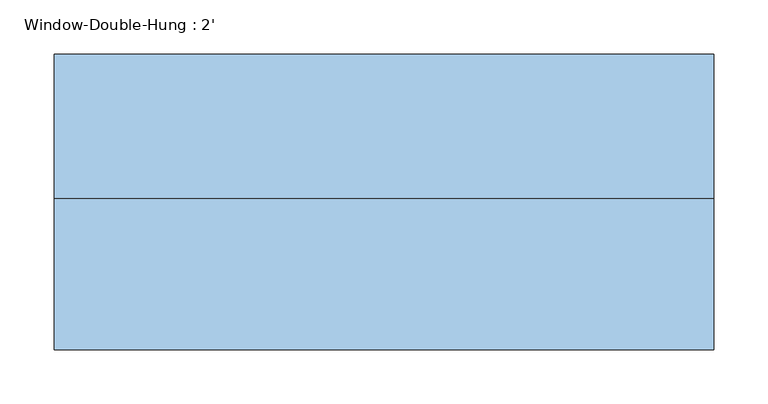
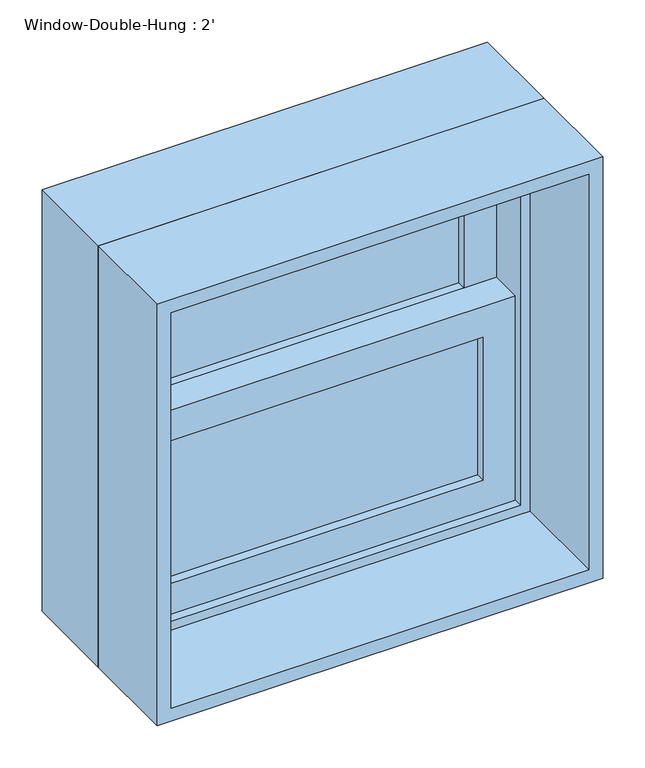
"""IFC4 building model written with IfcOpenShell, lengths in millimetres: window geometry, Window-Double-Hung : 2'."""

from ifc_helpers import new_model, si_unit, frame, origin, place, context, project, spatial, polyline, outline, extrude, source, transform, mapped, element, save


def window_double_hung_2_d0105baa(model_context):
    return source(origin(), model_context, "Body", "SweptSolid", [
        extrude(outline(polyline([(228.6, 57.15), (228.6, 50.8), (-228.6, 50.8), (-228.6, 57.15), (228.6, 57.15)])), frame((0.0, 0.0, 990.6), z_axis=(0.0, 0.0, 1.0), x_axis=(1.0, 0.0, 0.0)), (0.0, 0.0, 1.0), 206.375),
        extrude(outline(polyline([(-228.6, 44.45), (228.6, 44.45), (228.6, 38.1), (-228.6, 38.1), (-228.6, 44.45)])), frame((0.0, 0.0, 990.6), z_axis=(0.0, 0.0, 1.0), x_axis=(1.0, 0.0, 0.0)), (0.0, 0.0, 1.0), 206.375),
        extrude(outline(polyline([(228.6, 101.6), (228.6, 95.25), (-228.6, 95.25), (-228.6, 101.6), (228.6, 101.6)])), frame((0.0, 0.0, 1241.425), z_axis=(0.0, 0.0, 1.0), x_axis=(1.0, 0.0, 0.0)), (0.0, 0.0, 1.0), 206.375),
        extrude(outline(polyline([(-228.6, 88.9), (228.6, 88.9), (228.6, 82.55), (-228.6, 82.55), (-228.6, 88.9)])), frame((0.0, 0.0, 1241.425), z_axis=(0.0, 0.0, 1.0), x_axis=(1.0, 0.0, 0.0)), (0.0, 0.0, 1.0), 206.375),
        extrude(outline(polyline([(1241.425, -273.05), (946.15, -273.05), (946.15, 273.05), (1241.425, 273.05), (1241.425, -273.05)]), holes=[polyline([(1196.975, 228.6), (990.6, 228.6), (990.6, -228.6), (1196.975, -228.6), (1196.975, 228.6)])]), frame((0.0, 25.4, 0.0), z_axis=(0.0, 1.0, 0.0), x_axis=(0.0, 0.0, 1.0)), (0.0, 0.0, 1.0), 44.45),
        extrude(outline(polyline([(1492.25, -273.05), (1196.975, -273.05), (1196.975, 273.05), (1492.25, 273.05), (1492.25, -273.05)]), holes=[polyline([(1447.8, 228.6), (1241.425, 228.6), (1241.425, -228.6), (1447.8, -228.6), (1447.8, 228.6)])]), frame((0.0, 69.85, 0.0), z_axis=(0.0, 1.0, 0.0), x_axis=(0.0, 0.0, 1.0)), (0.0, 0.0, 1.0), 44.45),
        extrude(outline(polyline([(1524.0, -304.8), (914.4, -304.8), (914.4, 304.8), (1524.0, 304.8), (1524.0, -304.8)]), holes=[polyline([(1492.25, 273.05), (946.15, 273.05), (946.15, -273.05), (1492.25, -273.05), (1492.25, 273.05)])]), frame((0.0, 12.7, 0.0), z_axis=(0.0, 1.0, 0.0), x_axis=(0.0, 0.0, 1.0)), (0.0, 0.0, 1.0), 133.35),
        extrude(outline(polyline([(1524.0, 304.8), (1524.0, -304.8), (914.4, -304.8), (914.4, 304.8), (1524.0, 304.8)]), holes=[polyline([(1504.95, 285.75), (933.45, 285.75), (933.45, -285.75), (1504.95, -285.75), (1504.95, 285.75)])]), frame((0.0, -127.0, 0.0), z_axis=(0.0, 1.0, 0.0), x_axis=(0.0, 0.0, 1.0)), (0.0, 0.0, 1.0), 139.7),
    ])


if __name__ == "__main__":
    model = new_model("IFC4")
    model_context = context("Model", 3, world=origin())
    ifc_project = project(units=[si_unit("LENGTHUNIT", "METRE", prefix="MILLI")], contexts=[model_context])
    site = spatial("IfcSite", under=ifc_project)
    building = spatial("IfcBuilding", under=site)
    placement = place(None, origin())
    window_double_hung_2_shape = window_double_hung_2_d0105baa(model_context)
    element("IfcWindow", 1, ObjectType="Window-Double-Hung : 2'", at=placement, inside=building, context=model_context, shape_type="MappedRepresentation", body=[
        mapped(window_double_hung_2_shape, transform((0.0, 0.0, 0.0), x_axis=(1.0, 0.0, 0.0), y_axis=(0.0, 1.0, 0.0), z_axis=(0.0, 0.0, 1.0))),
    ])
    save(model, "model.ifc")

# Revit data of these elements
# Type "Window-Double-Hung : 2'"
#   Type Mark = "20"
#   Fire Rating = "0.5h"
#   Construction Type Id = "DG-DR"
#   Assembly Code = "B2020100"
#   Analytic Construction = "Double glazing - domestic"
#   Wall Thickness [instance default] = 0' - 6"
#   Window Inset [instance default] = 0' - 0"
#   Visual Light Transmittance = 0.81
#   Thermal Resistance (R) = 1.8146 (h·ft²·°F)/BTU
#   Solar Heat Gain Coefficient = 0.76
#   Muntin Width = 1' - 6"
#   Muntin Height = 0' - 8 1/8"
#   Interior Wall Closure [instance default] = 0' - 1 1/2"
#   Rough Width = 2' - 0 1/2"
#   Rough Height = 2' - 0 1/2"
#   Frame Extension [instance default] = 0' - 1 1/4"
#   Exterior Wall Closure [instance default] = 0' - 0 1/2"
#   Extension Jamb [instance default] = 0' - 1 1/2"
#   Heat Transfer Coefficient (U) = 0.5511 BTU/(h·ft²·°F)
#   Height = 2' - 0"
#   Width = 2' - 0"
#   Top Muntin Visibility = yes
#   Indicator Visibility [instance default] = yes
#   Extension Jamb Visibility [instance default] = yes
#   Interior Trim Visibility [instance default] = yes
#   Exterior Trim Visibility [instance default] = yes
#   Define Thermal Properties by = 1
#   Bottom Muntin Visibility = yes
#   Muntin Pattern = Muntin Pattern_2x2 : Muntin Pattern_2x2
#   Interior Trim Material = Wood - Stained
#   Interior Trim = Trim-Window-Interior-Flat : Picture Frame
#   Exterior Trim Material = Clad - White
#   Exterior Trim = Trim-Window-Exterior-Flat : with Sill
#   Glass Panel Material = Glass
#   Exterior Frame Material = Clad - White
#   Interior Frame Material = Wood - Stained
#   Wall Closure = (empty or 0)
# Element 1 (IfcWindow, "Window-Double-Hung : 2'")
#   Wall Thickness = 0' - 10"
#   Extension Jamb = 0' - 5 1/2"
#   Materials on its faces: "Wood - Stained", "Glass", "Clad - White"
# Materials
#   "Wood - Stained": class "Wood", colour RGB 224 178 126, transparency 0, Cost = 0
#   "Clad - White": class "Wood", colour RGB 242 242 238, transparency 0, Cost = 0
#   "Glass": class "Glass", colour RGB 0 128 192, transparency 0.75, Description = "Soda Lime Glass", Cost = 0
